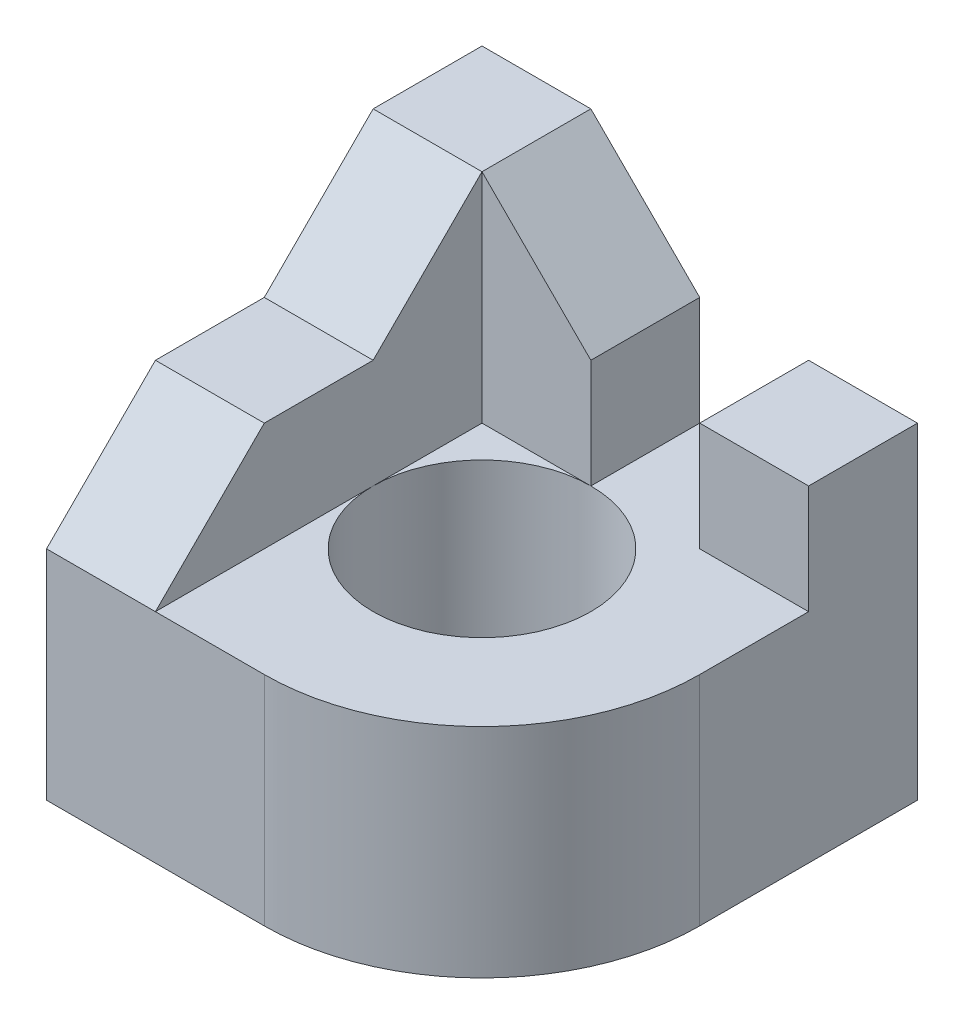
ISO-10303-21;
HEADER;
FILE_DESCRIPTION(('STEP AP214'),'2;1');
FILE_NAME('part.step','',(''),(''),'','','');
FILE_SCHEMA(('AUTOMOTIVE_DESIGN { 1 0 10303 214 1 1 1 1 }'));
ENDSEC;
DATA;
#1=APPLICATION_CONTEXT('core data for automotive mechanical design processes');
#2=APPLICATION_PROTOCOL_DEFINITION('international standard','automotive_design',2000,#1);
#3=PRODUCT_CONTEXT('',#1,'mechanical');
#4=PRODUCT('Part','Part','',(#3));
#5=PRODUCT_RELATED_PRODUCT_CATEGORY('part','',(#4));
#6=PRODUCT_DEFINITION_FORMATION('','',#4);
#7=PRODUCT_DEFINITION_CONTEXT('part definition',#1,'design');
#8=PRODUCT_DEFINITION('design','',#6,#7);
#9=PRODUCT_DEFINITION_SHAPE('','',#8);
#10=(LENGTH_UNIT() NAMED_UNIT(*) SI_UNIT(.MILLI.,.METRE.));
#11=(NAMED_UNIT(*) PLANE_ANGLE_UNIT() SI_UNIT($,.RADIAN.));
#12=(NAMED_UNIT(*) SI_UNIT($,.STERADIAN.) SOLID_ANGLE_UNIT());
#13=UNCERTAINTY_MEASURE_WITH_UNIT(LENGTH_MEASURE(1.E-05),#10,'distance_accuracy_value','');
#14=(GEOMETRIC_REPRESENTATION_CONTEXT(3) GLOBAL_UNCERTAINTY_ASSIGNED_CONTEXT((#13)) GLOBAL_UNIT_ASSIGNED_CONTEXT((#10,
#11,#12)) REPRESENTATION_CONTEXT('',''));
#15=CARTESIAN_POINT('',(0.,0.,0.));
#16=DIRECTION('',(0.,0.,1.));
#17=DIRECTION('',(1.,0.,0.));
#18=AXIS2_PLACEMENT_3D('',#15,#16,#17);
#19=CARTESIAN_POINT('',(0.,10.,0.));
#20=DIRECTION('',(0.,1.,0.));
#21=DIRECTION('',(0.,0.,1.));
#22=AXIS2_PLACEMENT_3D('',#19,#20,#21);
#23=PLANE('',#22);
#24=CARTESIAN_POINT('',(0.,10.,0.));
#25=DIRECTION('',(0.,1.,0.));
#26=DIRECTION('',(0.,0.,1.));
#27=AXIS2_PLACEMENT_3D('',#24,#25,#26);
#28=CIRCLE('',#27,10.);
#29=CARTESIAN_POINT('',(-10.,10.,0.));
#30=VERTEX_POINT('',#29);
#31=CARTESIAN_POINT('',(0.,10.,-10.));
#32=VERTEX_POINT('',#31);
#33=EDGE_CURVE('E54',#30,#32,#28,.F.);
#34=ORIENTED_EDGE('',*,*,#33,.T.);
#35=DIRECTION('',(1.,0.,0.));
#36=VECTOR('',#35,1.);
#37=CARTESIAN_POINT('',(0.,10.,-10.));
#38=LINE('',#37,#36);
#39=CARTESIAN_POINT('',(-10.,10.,-10.));
#40=VERTEX_POINT('',#39);
#41=EDGE_CURVE('E152',#40,#32,#38,.T.);
#42=ORIENTED_EDGE('',*,*,#41,.F.);
#43=DIRECTION('',(0.,0.,1.));
#44=VECTOR('',#43,1.);
#45=CARTESIAN_POINT('',(-10.,10.,-20.));
#46=LINE('',#45,#44);
#47=EDGE_CURVE('E156',#40,#30,#46,.T.);
#48=ORIENTED_EDGE('',*,*,#47,.T.);
#49=EDGE_LOOP('',(#34,#42,#48));
#50=FACE_BOUND('',#49,.T.);
#51=ADVANCED_FACE('F41',(#50),#23,.T.);
#52=CARTESIAN_POINT('',(-10.,0.,0.));
#53=DIRECTION('',(-1.,0.,0.));
#54=DIRECTION('',(0.,0.,1.));
#55=AXIS2_PLACEMENT_3D('',#52,#53,#54);
#56=PLANE('',#55);
#57=DIRECTION('',(0.,-1.,0.));
#58=VECTOR('',#57,1.);
#59=CARTESIAN_POINT('',(-10.,0.,-10.));
#60=LINE('',#59,#58);
#61=CARTESIAN_POINT('',(-10.,30.,-10.));
#62=VERTEX_POINT('',#61);
#63=EDGE_CURVE('E167',#62,#40,#60,.T.);
#64=ORIENTED_EDGE('',*,*,#63,.F.);
#65=DIRECTION('',(0.,0.707106781186548,-0.707106781186547));
#66=VECTOR('',#65,1.);
#67=CARTESIAN_POINT('',(-10.,30.,-10.));
#68=LINE('',#67,#66);
#69=CARTESIAN_POINT('',(-10.,20.,0.));
#70=VERTEX_POINT('',#69);
#71=EDGE_CURVE('E197',#70,#62,#68,.T.);
#72=ORIENTED_EDGE('',*,*,#71,.F.);
#73=DIRECTION('',(0.,0.,-1.));
#74=VECTOR('',#73,1.);
#75=CARTESIAN_POINT('',(-10.,20.,0.));
#76=LINE('',#75,#74);
#77=CARTESIAN_POINT('',(-10.,20.,10.));
#78=VERTEX_POINT('',#77);
#79=EDGE_CURVE('E191',#78,#70,#76,.T.);
#80=ORIENTED_EDGE('',*,*,#79,.F.);
#81=DIRECTION('',(0.,0.707106781186548,-0.707106781186548));
#82=VECTOR('',#81,1.);
#83=CARTESIAN_POINT('',(-10.,20.,10.));
#84=LINE('',#83,#82);
#85=CARTESIAN_POINT('',(-10.,10.,20.));
#86=VERTEX_POINT('',#85);
#87=EDGE_CURVE('E192',#86,#78,#84,.T.);
#88=ORIENTED_EDGE('',*,*,#87,.F.);
#89=EDGE_CURVE('E62',#30,#86,#46,.T.);
#90=ORIENTED_EDGE('',*,*,#89,.F.);
#91=ORIENTED_EDGE('',*,*,#47,.F.);
#92=EDGE_LOOP('',(#64,#72,#80,#88,#90,#91));
#93=FACE_BOUND('',#92,.T.);
#94=ADVANCED_FACE('F312',(#93),#56,.F.);
#95=EDGE_CURVE('E144',#32,#30,#28,.F.);
#96=ORIENTED_EDGE('',*,*,#95,.T.);
#97=ORIENTED_EDGE('',*,*,#89,.T.);
#98=DIRECTION('',(1.,0.,0.));
#99=VECTOR('',#98,1.);
#100=CARTESIAN_POINT('',(-1.45716771982052E-13,10.,20.));
#101=LINE('',#100,#99);
#102=CARTESIAN_POINT('',(-1.45577994103974E-13,10.,20.));
#103=VERTEX_POINT('',#102);
#104=EDGE_CURVE('E246',#86,#103,#101,.T.);
#105=ORIENTED_EDGE('',*,*,#104,.T.);
#106=CARTESIAN_POINT('',(0.,10.,0.));
#107=DIRECTION('',(0.,1.,0.));
#108=DIRECTION('',(0.,0.,1.));
#109=AXIS2_PLACEMENT_3D('',#106,#107,#108);
#110=CIRCLE('',#109,20.);
#111=CARTESIAN_POINT('',(20.,10.,-1.52655665885959E-13));
#112=VERTEX_POINT('',#111);
#113=EDGE_CURVE('E249',#103,#112,#110,.T.);
#114=ORIENTED_EDGE('',*,*,#113,.T.);
#115=DIRECTION('',(0.,0.,-1.));
#116=VECTOR('',#115,1.);
#117=CARTESIAN_POINT('',(20.,10.,-1.52655665885959E-13));
#118=LINE('',#117,#116);
#119=CARTESIAN_POINT('',(20.,10.,-10.));
#120=VERTEX_POINT('',#119);
#121=EDGE_CURVE('E253',#112,#120,#118,.T.);
#122=ORIENTED_EDGE('',*,*,#121,.T.);
#123=DIRECTION('',(1.,0.,0.));
#124=VECTOR('',#123,1.);
#125=CARTESIAN_POINT('',(20.,10.,-10.));
#126=LINE('',#125,#124);
#127=CARTESIAN_POINT('',(10.,10.,-10.));
#128=VERTEX_POINT('',#127);
#129=EDGE_CURVE('E223',#128,#120,#126,.T.);
#130=ORIENTED_EDGE('',*,*,#129,.F.);
#131=DIRECTION('',(0.,0.,1.));
#132=VECTOR('',#131,1.);
#133=CARTESIAN_POINT('',(10.,10.,-20.));
#134=LINE('',#133,#132);
#135=CARTESIAN_POINT('',(10.,10.,-20.));
#136=VERTEX_POINT('',#135);
#137=EDGE_CURVE('E214',#136,#128,#134,.T.);
#138=ORIENTED_EDGE('',*,*,#137,.F.);
#139=DIRECTION('',(-1.,0.,0.));
#140=VECTOR('',#139,1.);
#141=CARTESIAN_POINT('',(20.,10.,-20.));
#142=LINE('',#141,#140);
#143=CARTESIAN_POINT('',(2.20427223898739E-13,10.,-20.));
#144=VERTEX_POINT('',#143);
#145=EDGE_CURVE('E176',#136,#144,#142,.T.);
#146=ORIENTED_EDGE('',*,*,#145,.T.);
#147=DIRECTION('',(0.,0.,-1.));
#148=VECTOR('',#147,1.);
#149=CARTESIAN_POINT('',(2.22161947374716E-13,10.,-10.));
#150=LINE('',#149,#148);
#151=EDGE_CURVE('E171',#32,#144,#150,.T.);
#152=ORIENTED_EDGE('',*,*,#151,.F.);
#153=EDGE_LOOP('',(#96,#97,#105,#114,#122,#130,#138,#146,#152));
#154=FACE_BOUND('',#153,.T.);
#155=ADVANCED_FACE('F180',(#154),#23,.T.);
#156=CARTESIAN_POINT('',(-20.,10.,20.));
#157=DIRECTION('',(1.,0.,0.));
#158=DIRECTION('',(0.,0.,-1.));
#159=AXIS2_PLACEMENT_3D('',#156,#157,#158);
#160=PLANE('',#159);
#161=DIRECTION('',(0.,0.,1.));
#162=VECTOR('',#161,1.);
#163=CARTESIAN_POINT('',(-20.,-10.,20.));
#164=LINE('',#163,#162);
#165=CARTESIAN_POINT('',(-20.,-10.,-20.));
#166=VERTEX_POINT('',#165);
#167=CARTESIAN_POINT('',(-20.,-10.,20.));
#168=VERTEX_POINT('',#167);
#169=EDGE_CURVE('E243',#166,#168,#164,.T.);
#170=ORIENTED_EDGE('',*,*,#169,.T.);
#171=DIRECTION('',(0.,-1.,0.));
#172=VECTOR('',#171,1.);
#173=CARTESIAN_POINT('',(-20.,10.,20.));
#174=LINE('',#173,#172);
#175=CARTESIAN_POINT('',(-20.,10.,20.));
#176=VERTEX_POINT('',#175);
#177=EDGE_CURVE('E11',#176,#168,#174,.T.);
#178=ORIENTED_EDGE('',*,*,#177,.F.);
#179=DIRECTION('',(0.,0.707106781186548,-0.707106781186548));
#180=VECTOR('',#179,1.);
#181=CARTESIAN_POINT('',(-20.,20.,10.));
#182=LINE('',#181,#180);
#183=CARTESIAN_POINT('',(-20.,20.,10.));
#184=VERTEX_POINT('',#183);
#185=EDGE_CURVE('E178',#176,#184,#182,.T.);
#186=ORIENTED_EDGE('',*,*,#185,.T.);
#187=DIRECTION('',(0.,0.,-1.));
#188=VECTOR('',#187,1.);
#189=CARTESIAN_POINT('',(-20.,20.,0.));
#190=LINE('',#189,#188);
#191=CARTESIAN_POINT('',(-20.,20.,0.));
#192=VERTEX_POINT('',#191);
#193=EDGE_CURVE('E181',#184,#192,#190,.T.);
#194=ORIENTED_EDGE('',*,*,#193,.T.);
#195=DIRECTION('',(0.,0.707106781186548,-0.707106781186547));
#196=VECTOR('',#195,1.);
#197=CARTESIAN_POINT('',(-20.,30.,-10.));
#198=LINE('',#197,#196);
#199=CARTESIAN_POINT('',(-20.,30.,-10.));
#200=VERTEX_POINT('',#199);
#201=EDGE_CURVE('E206',#192,#200,#198,.T.);
#202=ORIENTED_EDGE('',*,*,#201,.T.);
#203=DIRECTION('',(0.,0.,-1.));
#204=VECTOR('',#203,1.);
#205=CARTESIAN_POINT('',(-20.,30.,-20.));
#206=LINE('',#205,#204);
#207=CARTESIAN_POINT('',(-20.,30.,-20.));
#208=VERTEX_POINT('',#207);
#209=EDGE_CURVE('E207',#200,#208,#206,.T.);
#210=ORIENTED_EDGE('',*,*,#209,.T.);
#211=DIRECTION('',(0.,-1.,0.));
#212=VECTOR('',#211,1.);
#213=CARTESIAN_POINT('',(-20.,10.,-20.));
#214=LINE('',#213,#212);
#215=EDGE_CURVE('E255',#208,#166,#214,.T.);
#216=ORIENTED_EDGE('',*,*,#215,.T.);
#217=EDGE_LOOP('',(#170,#178,#186,#194,#202,#210,#216));
#218=FACE_BOUND('',#217,.T.);
#219=ADVANCED_FACE('F43',(#218),#160,.F.);
#220=CARTESIAN_POINT('',(-1.45716771982052E-13,10.,20.));
#221=DIRECTION('',(0.,0.,-1.));
#222=DIRECTION('',(-1.,0.,0.));
#223=AXIS2_PLACEMENT_3D('',#220,#221,#222);
#224=PLANE('',#223);
#225=DIRECTION('',(1.,0.,0.));
#226=VECTOR('',#225,1.);
#227=CARTESIAN_POINT('',(-1.45716771982052E-13,-10.,20.));
#228=LINE('',#227,#226);
#229=CARTESIAN_POINT('',(-1.45577994103974E-13,-10.,20.));
#230=VERTEX_POINT('',#229);
#231=EDGE_CURVE('E260',#168,#230,#228,.T.);
#232=ORIENTED_EDGE('',*,*,#231,.T.);
#233=DIRECTION('',(0.,-1.,0.));
#234=VECTOR('',#233,1.);
#235=CARTESIAN_POINT('',(-1.45577994103974E-13,10.,20.));
#236=LINE('',#235,#234);
#237=EDGE_CURVE('E47',#103,#230,#236,.T.);
#238=ORIENTED_EDGE('',*,*,#237,.F.);
#239=ORIENTED_EDGE('',*,*,#104,.F.);
#240=EDGE_CURVE('E245',#176,#86,#101,.T.);
#241=ORIENTED_EDGE('',*,*,#240,.F.);
#242=ORIENTED_EDGE('',*,*,#177,.T.);
#243=EDGE_LOOP('',(#232,#238,#239,#241,#242));
#244=FACE_BOUND('',#243,.T.);
#245=ADVANCED_FACE('F326',(#244),#224,.F.);
#246=CARTESIAN_POINT('',(0.,10.,0.));
#247=DIRECTION('',(0.,-1.,0.));
#248=DIRECTION('',(0.,0.,-1.));
#249=AXIS2_PLACEMENT_3D('',#246,#247,#248);
#250=CYLINDRICAL_SURFACE('',#249,20.);
#251=CARTESIAN_POINT('',(0.,-10.,0.));
#252=DIRECTION('',(0.,1.,0.));
#253=DIRECTION('',(0.,0.,1.));
#254=AXIS2_PLACEMENT_3D('',#251,#252,#253);
#255=CIRCLE('',#254,20.);
#256=CARTESIAN_POINT('',(20.,-10.,-1.52655665885959E-13));
#257=VERTEX_POINT('',#256);
#258=EDGE_CURVE('E259',#230,#257,#255,.T.);
#259=ORIENTED_EDGE('',*,*,#258,.T.);
#260=DIRECTION('',(0.,-1.,0.));
#261=VECTOR('',#260,1.);
#262=CARTESIAN_POINT('',(20.,10.,-1.52655665885959E-13));
#263=LINE('',#262,#261);
#264=EDGE_CURVE('E269',#112,#257,#263,.T.);
#265=ORIENTED_EDGE('',*,*,#264,.F.);
#266=ORIENTED_EDGE('',*,*,#113,.F.);
#267=ORIENTED_EDGE('',*,*,#237,.T.);
#268=EDGE_LOOP('',(#259,#265,#266,#267));
#269=FACE_BOUND('',#268,.T.);
#270=ADVANCED_FACE('F280',(#269),#250,.T.);
#271=CARTESIAN_POINT('',(20.,10.,-1.52655665885959E-13));
#272=DIRECTION('',(-1.,0.,0.));
#273=DIRECTION('',(0.,0.,1.));
#274=AXIS2_PLACEMENT_3D('',#271,#272,#273);
#275=PLANE('',#274);
#276=DIRECTION('',(0.,0.,-1.));
#277=VECTOR('',#276,1.);
#278=CARTESIAN_POINT('',(20.,-10.,-1.52655665885959E-13));
#279=LINE('',#278,#277);
#280=CARTESIAN_POINT('',(20.,-10.,-20.));
#281=VERTEX_POINT('',#280);
#282=EDGE_CURVE('E261',#257,#281,#279,.T.);
#283=ORIENTED_EDGE('',*,*,#282,.T.);
#284=DIRECTION('',(0.,-1.,0.));
#285=VECTOR('',#284,1.);
#286=CARTESIAN_POINT('',(20.,10.,-20.));
#287=LINE('',#286,#285);
#288=CARTESIAN_POINT('',(20.,20.,-20.));
#289=VERTEX_POINT('',#288);
#290=EDGE_CURVE('E270',#289,#281,#287,.T.);
#291=ORIENTED_EDGE('',*,*,#290,.F.);
#292=DIRECTION('',(0.,0.,-1.));
#293=VECTOR('',#292,1.);
#294=CARTESIAN_POINT('',(20.,20.,-20.));
#295=LINE('',#294,#293);
#296=CARTESIAN_POINT('',(20.,20.,-10.));
#297=VERTEX_POINT('',#296);
#298=EDGE_CURVE('E222',#297,#289,#295,.T.);
#299=ORIENTED_EDGE('',*,*,#298,.F.);
#300=DIRECTION('',(0.,-1.,0.));
#301=VECTOR('',#300,1.);
#302=CARTESIAN_POINT('',(20.,20.,-10.));
#303=LINE('',#302,#301);
#304=EDGE_CURVE('E232',#297,#120,#303,.T.);
#305=ORIENTED_EDGE('',*,*,#304,.T.);
#306=ORIENTED_EDGE('',*,*,#121,.F.);
#307=ORIENTED_EDGE('',*,*,#264,.T.);
#308=EDGE_LOOP('',(#283,#291,#299,#305,#306,#307));
#309=FACE_BOUND('',#308,.T.);
#310=ADVANCED_FACE('F287',(#309),#275,.F.);
#311=CARTESIAN_POINT('',(20.,10.,-20.));
#312=DIRECTION('',(0.,0.,1.));
#313=DIRECTION('',(1.,0.,0.));
#314=AXIS2_PLACEMENT_3D('',#311,#312,#313);
#315=PLANE('',#314);
#316=DIRECTION('',(0.,-1.,0.));
#317=VECTOR('',#316,1.);
#318=CARTESIAN_POINT('',(0.,0.,-20.));
#319=LINE('',#318,#317);
#320=CARTESIAN_POINT('',(0.,19.9999999999998,-20.));
#321=VERTEX_POINT('',#320);
#322=EDGE_CURVE('E187',#321,#144,#319,.T.);
#323=ORIENTED_EDGE('',*,*,#322,.T.);
#324=ORIENTED_EDGE('',*,*,#145,.F.);
#325=DIRECTION('',(0.,-1.,0.));
#326=VECTOR('',#325,1.);
#327=CARTESIAN_POINT('',(10.,20.,-20.));
#328=LINE('',#327,#326);
#329=CARTESIAN_POINT('',(10.,20.,-20.));
#330=VERTEX_POINT('',#329);
#331=EDGE_CURVE('E241',#330,#136,#328,.T.);
#332=ORIENTED_EDGE('',*,*,#331,.F.);
#333=DIRECTION('',(-1.,0.,0.));
#334=VECTOR('',#333,1.);
#335=CARTESIAN_POINT('',(20.,20.,-20.));
#336=LINE('',#335,#334);
#337=EDGE_CURVE('E221',#289,#330,#336,.T.);
#338=ORIENTED_EDGE('',*,*,#337,.F.);
#339=ORIENTED_EDGE('',*,*,#290,.T.);
#340=DIRECTION('',(-1.,0.,0.));
#341=VECTOR('',#340,1.);
#342=CARTESIAN_POINT('',(20.,-10.,-20.));
#343=LINE('',#342,#341);
#344=EDGE_CURVE('E263',#281,#166,#343,.T.);
#345=ORIENTED_EDGE('',*,*,#344,.T.);
#346=ORIENTED_EDGE('',*,*,#215,.F.);
#347=DIRECTION('',(-1.,0.,0.));
#348=VECTOR('',#347,1.);
#349=CARTESIAN_POINT('',(-10.,30.,-20.));
#350=LINE('',#349,#348);
#351=CARTESIAN_POINT('',(-10.,30.,-20.));
#352=VERTEX_POINT('',#351);
#353=EDGE_CURVE('E215',#352,#208,#350,.T.);
#354=ORIENTED_EDGE('',*,*,#353,.F.);
#355=DIRECTION('',(0.707106781186541,-0.707106781186554,0.));
#356=VECTOR('',#355,1.);
#357=CARTESIAN_POINT('',(9.99999999999991,9.99999999999974,-20.));
#358=LINE('',#357,#356);
#359=EDGE_CURVE('E160',#352,#321,#358,.T.);
#360=ORIENTED_EDGE('',*,*,#359,.T.);
#361=EDGE_LOOP('',(#323,#324,#332,#338,#339,#345,#346,#354,#360));
#362=FACE_BOUND('',#361,.T.);
#363=ADVANCED_FACE('F292',(#362),#315,.F.);
#364=CARTESIAN_POINT('',(0.,-10.,0.));
#365=DIRECTION('',(0.,1.,0.));
#366=DIRECTION('',(0.,0.,1.));
#367=AXIS2_PLACEMENT_3D('',#364,#365,#366);
#368=PLANE('',#367);
#369=CARTESIAN_POINT('',(0.,-10.,0.));
#370=DIRECTION('',(0.,-1.,0.));
#371=DIRECTION('',(0.,0.,-1.));
#372=AXIS2_PLACEMENT_3D('',#369,#370,#371);
#373=CIRCLE('',#372,10.);
#374=CARTESIAN_POINT('',(0.,-10.,-10.));
#375=VERTEX_POINT('',#374);
#376=EDGE_CURVE('E146',#375,#375,#373,.T.);
#377=ORIENTED_EDGE('',*,*,#376,.F.);
#378=EDGE_LOOP('',(#377));
#379=FACE_BOUND('',#378,.T.);
#380=ORIENTED_EDGE('',*,*,#169,.F.);
#381=ORIENTED_EDGE('',*,*,#344,.F.);
#382=ORIENTED_EDGE('',*,*,#282,.F.);
#383=ORIENTED_EDGE('',*,*,#258,.F.);
#384=ORIENTED_EDGE('',*,*,#231,.F.);
#385=EDGE_LOOP('',(#380,#381,#382,#383,#384));
#386=FACE_BOUND('',#385,.T.);
#387=ADVANCED_FACE('F284',(#379,#386),#368,.F.);
#388=CARTESIAN_POINT('',(10.,20.,-20.));
#389=DIRECTION('',(1.,0.,0.));
#390=DIRECTION('',(0.,0.,-1.));
#391=AXIS2_PLACEMENT_3D('',#388,#389,#390);
#392=PLANE('',#391);
#393=ORIENTED_EDGE('',*,*,#137,.T.);
#394=DIRECTION('',(0.,-1.,0.));
#395=VECTOR('',#394,1.);
#396=CARTESIAN_POINT('',(10.,20.,-10.));
#397=LINE('',#396,#395);
#398=CARTESIAN_POINT('',(10.,20.,-10.));
#399=VERTEX_POINT('',#398);
#400=EDGE_CURVE('E236',#399,#128,#397,.T.);
#401=ORIENTED_EDGE('',*,*,#400,.F.);
#402=DIRECTION('',(0.,0.,1.));
#403=VECTOR('',#402,1.);
#404=CARTESIAN_POINT('',(10.,20.,-20.));
#405=LINE('',#404,#403);
#406=EDGE_CURVE('E227',#330,#399,#405,.T.);
#407=ORIENTED_EDGE('',*,*,#406,.F.);
#408=ORIENTED_EDGE('',*,*,#331,.T.);
#409=EDGE_LOOP('',(#393,#401,#407,#408));
#410=FACE_BOUND('',#409,.T.);
#411=ADVANCED_FACE('F305',(#410),#392,.F.);
#412=CARTESIAN_POINT('',(20.,20.,-10.));
#413=DIRECTION('',(0.,0.,-1.));
#414=DIRECTION('',(-1.,0.,0.));
#415=AXIS2_PLACEMENT_3D('',#412,#413,#414);
#416=PLANE('',#415);
#417=ORIENTED_EDGE('',*,*,#129,.T.);
#418=ORIENTED_EDGE('',*,*,#304,.F.);
#419=DIRECTION('',(1.,0.,0.));
#420=VECTOR('',#419,1.);
#421=CARTESIAN_POINT('',(20.,20.,-10.));
#422=LINE('',#421,#420);
#423=EDGE_CURVE('E228',#399,#297,#422,.T.);
#424=ORIENTED_EDGE('',*,*,#423,.F.);
#425=ORIENTED_EDGE('',*,*,#400,.T.);
#426=EDGE_LOOP('',(#417,#418,#424,#425));
#427=FACE_BOUND('',#426,.T.);
#428=ADVANCED_FACE('F298',(#427),#416,.F.);
#429=CARTESIAN_POINT('',(0.,20.,0.));
#430=DIRECTION('',(0.,-1.,0.));
#431=DIRECTION('',(0.,0.,-1.));
#432=AXIS2_PLACEMENT_3D('',#429,#430,#431);
#433=PLANE('',#432);
#434=ORIENTED_EDGE('',*,*,#298,.T.);
#435=ORIENTED_EDGE('',*,*,#337,.T.);
#436=ORIENTED_EDGE('',*,*,#406,.T.);
#437=ORIENTED_EDGE('',*,*,#423,.T.);
#438=EDGE_LOOP('',(#434,#435,#436,#437));
#439=FACE_BOUND('',#438,.T.);
#440=ADVANCED_FACE('F293',(#439),#433,.F.);
#441=CARTESIAN_POINT('',(-10.,30.,-20.));
#442=DIRECTION('',(0.,1.,0.));
#443=DIRECTION('',(0.,0.,1.));
#444=AXIS2_PLACEMENT_3D('',#441,#442,#443);
#445=PLANE('',#444);
#446=ORIENTED_EDGE('',*,*,#209,.F.);
#447=DIRECTION('',(-1.,0.,0.));
#448=VECTOR('',#447,1.);
#449=CARTESIAN_POINT('',(-10.,30.,-10.));
#450=LINE('',#449,#448);
#451=EDGE_CURVE('E216',#62,#200,#450,.T.);
#452=ORIENTED_EDGE('',*,*,#451,.F.);
#453=DIRECTION('',(0.,0.,-1.));
#454=VECTOR('',#453,1.);
#455=CARTESIAN_POINT('',(-10.,30.,-20.));
#456=LINE('',#455,#454);
#457=EDGE_CURVE('E199',#62,#352,#456,.T.);
#458=ORIENTED_EDGE('',*,*,#457,.T.);
#459=ORIENTED_EDGE('',*,*,#353,.T.);
#460=EDGE_LOOP('',(#446,#452,#458,#459));
#461=FACE_BOUND('',#460,.T.);
#462=ADVANCED_FACE('F337',(#461),#445,.T.);
#463=CARTESIAN_POINT('',(-10.,30.,-10.));
#464=DIRECTION('',(0.,0.707106781186547,0.707106781186548));
#465=DIRECTION('',(0.,-0.707106781186548,0.707106781186547));
#466=AXIS2_PLACEMENT_3D('',#463,#464,#465);
#467=PLANE('',#466);
#468=ORIENTED_EDGE('',*,*,#201,.F.);
#469=DIRECTION('',(-1.,0.,0.));
#470=VECTOR('',#469,1.);
#471=CARTESIAN_POINT('',(-10.,20.,0.));
#472=LINE('',#471,#470);
#473=EDGE_CURVE('E217',#70,#192,#472,.T.);
#474=ORIENTED_EDGE('',*,*,#473,.F.);
#475=ORIENTED_EDGE('',*,*,#71,.T.);
#476=ORIENTED_EDGE('',*,*,#451,.T.);
#477=EDGE_LOOP('',(#468,#474,#475,#476));
#478=FACE_BOUND('',#477,.T.);
#479=ADVANCED_FACE('F362',(#478),#467,.T.);
#480=CARTESIAN_POINT('',(-10.,20.,0.));
#481=DIRECTION('',(0.,1.,0.));
#482=DIRECTION('',(0.,0.,1.));
#483=AXIS2_PLACEMENT_3D('',#480,#481,#482);
#484=PLANE('',#483);
#485=ORIENTED_EDGE('',*,*,#193,.F.);
#486=DIRECTION('',(-1.,0.,0.));
#487=VECTOR('',#486,1.);
#488=CARTESIAN_POINT('',(-10.,20.,10.));
#489=LINE('',#488,#487);
#490=EDGE_CURVE('E205',#78,#184,#489,.T.);
#491=ORIENTED_EDGE('',*,*,#490,.F.);
#492=ORIENTED_EDGE('',*,*,#79,.T.);
#493=ORIENTED_EDGE('',*,*,#473,.T.);
#494=EDGE_LOOP('',(#485,#491,#492,#493));
#495=FACE_BOUND('',#494,.T.);
#496=ADVANCED_FACE('F364',(#495),#484,.T.);
#497=CARTESIAN_POINT('',(-10.,20.,10.));
#498=DIRECTION('',(0.,0.707106781186548,0.707106781186548));
#499=DIRECTION('',(0.,-0.707106781186548,0.707106781186548));
#500=AXIS2_PLACEMENT_3D('',#497,#498,#499);
#501=PLANE('',#500);
#502=ORIENTED_EDGE('',*,*,#185,.F.);
#503=ORIENTED_EDGE('',*,*,#240,.T.);
#504=ORIENTED_EDGE('',*,*,#87,.T.);
#505=ORIENTED_EDGE('',*,*,#490,.T.);
#506=EDGE_LOOP('',(#502,#503,#504,#505));
#507=FACE_BOUND('',#506,.T.);
#508=ADVANCED_FACE('F359',(#507),#501,.T.);
#509=CARTESIAN_POINT('',(9.99999999999991,9.99999999999974,-10.));
#510=DIRECTION('',(0.707106781186554,0.707106781186541,0.));
#511=DIRECTION('',(-0.707106781186541,0.707106781186554,0.));
#512=AXIS2_PLACEMENT_3D('',#509,#510,#511);
#513=PLANE('',#512);
#514=ORIENTED_EDGE('',*,*,#359,.F.);
#515=ORIENTED_EDGE('',*,*,#457,.F.);
#516=DIRECTION('',(0.707106781186541,-0.707106781186554,0.));
#517=VECTOR('',#516,1.);
#518=CARTESIAN_POINT('',(9.99999999999991,9.99999999999974,-10.));
#519=LINE('',#518,#517);
#520=CARTESIAN_POINT('',(0.,19.9999999999998,-10.));
#521=VERTEX_POINT('',#520);
#522=EDGE_CURVE('E173',#62,#521,#519,.T.);
#523=ORIENTED_EDGE('',*,*,#522,.T.);
#524=DIRECTION('',(0.,0.,-1.));
#525=VECTOR('',#524,1.);
#526=CARTESIAN_POINT('',(0.,19.9999999999998,-10.));
#527=LINE('',#526,#525);
#528=EDGE_CURVE('E174',#521,#321,#527,.T.);
#529=ORIENTED_EDGE('',*,*,#528,.T.);
#530=EDGE_LOOP('',(#514,#515,#523,#529));
#531=FACE_BOUND('',#530,.T.);
#532=ADVANCED_FACE('F340',(#531),#513,.T.);
#533=CARTESIAN_POINT('',(0.,0.,-10.));
#534=DIRECTION('',(1.,0.,0.));
#535=DIRECTION('',(0.,1.,0.));
#536=AXIS2_PLACEMENT_3D('',#533,#534,#535);
#537=PLANE('',#536);
#538=ORIENTED_EDGE('',*,*,#322,.F.);
#539=ORIENTED_EDGE('',*,*,#528,.F.);
#540=DIRECTION('',(0.,-1.,0.));
#541=VECTOR('',#540,1.);
#542=CARTESIAN_POINT('',(0.,0.,-10.));
#543=LINE('',#542,#541);
#544=EDGE_CURVE('E162',#521,#32,#543,.T.);
#545=ORIENTED_EDGE('',*,*,#544,.T.);
#546=ORIENTED_EDGE('',*,*,#151,.T.);
#547=EDGE_LOOP('',(#538,#539,#545,#546));
#548=FACE_BOUND('',#547,.T.);
#549=ADVANCED_FACE('F168',(#548),#537,.T.);
#550=CARTESIAN_POINT('',(0.,0.,-10.));
#551=DIRECTION('',(0.,0.,-1.));
#552=DIRECTION('',(-1.,0.,0.));
#553=AXIS2_PLACEMENT_3D('',#550,#551,#552);
#554=PLANE('',#553);
#555=ORIENTED_EDGE('',*,*,#522,.F.);
#556=ORIENTED_EDGE('',*,*,#63,.T.);
#557=ORIENTED_EDGE('',*,*,#41,.T.);
#558=ORIENTED_EDGE('',*,*,#544,.F.);
#559=EDGE_LOOP('',(#555,#556,#557,#558));
#560=FACE_BOUND('',#559,.T.);
#561=ADVANCED_FACE('F165',(#560),#554,.F.);
#562=CARTESIAN_POINT('',(0.,38.2842712474619,0.));
#563=DIRECTION('',(0.,-1.,0.));
#564=DIRECTION('',(0.,0.,-1.));
#565=AXIS2_PLACEMENT_3D('',#562,#563,#564);
#566=CYLINDRICAL_SURFACE('',#565,10.);
#567=ORIENTED_EDGE('',*,*,#376,.T.);
#568=EDGE_LOOP('',(#567));
#569=FACE_BOUND('',#568,.T.);
#570=ORIENTED_EDGE('',*,*,#33,.F.);
#571=ORIENTED_EDGE('',*,*,#95,.F.);
#572=EDGE_LOOP('',(#570,#571));
#573=FACE_BOUND('',#572,.T.);
#574=ADVANCED_FACE('F148',(#569,#573),#566,.F.);
#575=CLOSED_SHELL('',(#51,#94,#155,#219,#245,#270,#310,#363,#387,#411,#428,#440,#462,#479,#496,
#508,#532,#549,#561,#574));
#576=MANIFOLD_SOLID_BREP('B2',#575);
#577=ADVANCED_BREP_SHAPE_REPRESENTATION('',(#18,#576),#14);
#578=SHAPE_DEFINITION_REPRESENTATION(#9,#577);
ENDSEC;
END-ISO-10303-21;
